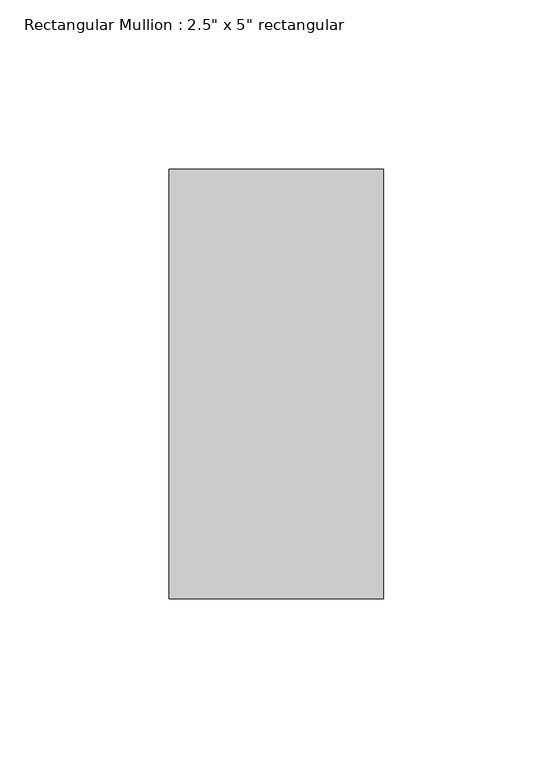
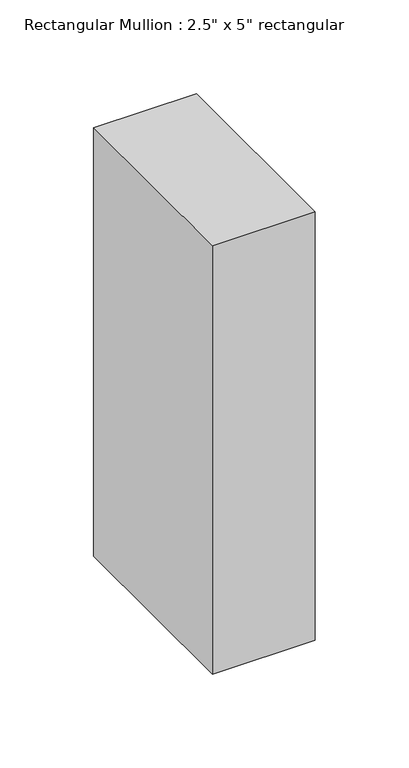
"""IFC4 building model written with IfcOpenShell, lengths in millimetres: member geometry."""

from ifc_helpers import new_model, si_unit, frame, origin, place, context, project, spatial, polyline, outline, extrude, source, transform, mapped, element, save


def member_6be37683(model_context):
    return source(origin(), model_context, "Body", "SweptSolid", [
        extrude(outline(polyline([(31.75, 63.5), (31.75, -63.5), (-31.75, -63.5), (-31.75, 63.5), (31.75, 63.5)])), frame((0.0, 0.0, -279.4), z_axis=(0.0, 0.0, 1.0), x_axis=(1.0, 0.0, 0.0)), (0.0, 0.0, 1.0), 279.4),
    ])


if __name__ == "__main__":
    model = new_model("IFC4")
    model_context = context("Model", 3, world=origin())
    ifc_project = project(units=[si_unit("LENGTHUNIT", "METRE", prefix="MILLI")], contexts=[model_context])
    site = spatial("IfcSite", under=ifc_project)
    building = spatial("IfcBuilding", under=site)
    placement = place(None, origin())
    member_shape = member_6be37683(model_context)
    element("IfcMember", 1, ObjectType="Rectangular Mullion : 2.5\" x 5\" rectangular", at=placement, inside=building, context=model_context, shape_type="MappedRepresentation", body=[
        mapped(member_shape, transform((0.0, 0.0, 0.0), x_axis=(1.0, 0.0, 0.0), y_axis=(0.0, 1.0, 0.0), z_axis=(0.0, 0.0, 1.0))),
    ])
    save(model, "model.ifc")

# Revit data of these elements
# Type "Rectangular Mullion : 2.5\" x 5\" rectangular"
#   built-in parameter 1007304 = 0.416667 (stored number, unit not read)
#   built-in parameter 1007301 = 0.104167 (stored number, unit not read)
#   built-in parameter 1007300 = 0.104167 (stored number, unit not read)
